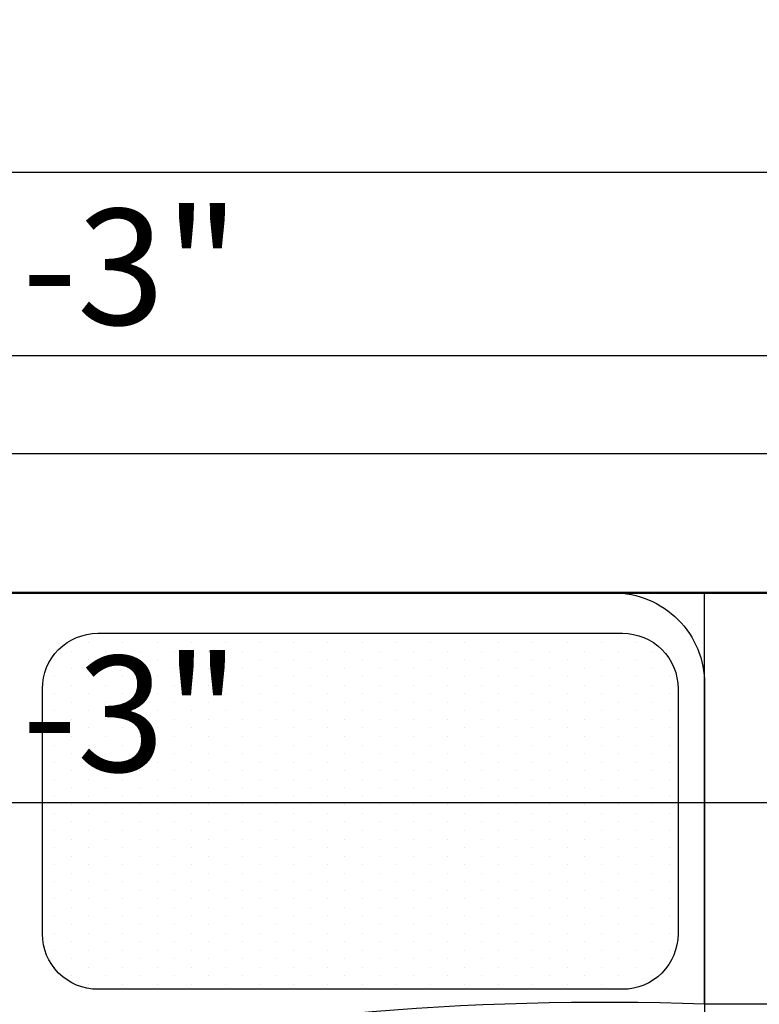
# Model space of a CAD drawing. Units: inches. Extents: x 3064 to 19385, y 846 to 15425.
# Tile 90 of 108: x 7338 to 7370, y 1373 to 1415. Entities that reach past the tile are written whole.
import ezdxf

# ---------------------------------------------------------------- set-up
doc = ezdxf.new("R2010")
doc.units = ezdxf.units.IN
for name, color, linetype, lineweight in [('A-ANNO-DIMS', 2, 'Continuous', 18), ('A-FLOR-FIXT', 9, 'Continuous', 18), ('A-WALL', 7, 'Continuous', 50), ('C-PROP', 6, 'Continuous', 25)]:
    doc.layers.add(name, color=color, linetype=linetype, lineweight=lineweight)
doc.layers.add('BLOCK', color=6, linetype='Continuous')
doc.styles.get("Standard").update_dxf_attribs({"font": 'arial.ttf'})
doc.dimstyles.new('ISO-25', dxfattribs={"dimtxt": 9, "dimasz": 2.5, "dimexe": 1.25, "dimexo": 0.625, "dimtad": 1, "dimdec": 1, "dimlunit": 3, "dimtxsty": 'Standard', "dimcen": 2.5, "dimadec": 0, "dimazin": 0, "dimtfac": 1, "dimtdec": 1, "dimtmove": 0, "dimatfit": 3, "dimfxl": 1, "dimarcsym": 0})

# ---------------------------------------------------------------- blocks, each defined once
blk = doc.blocks.new('*D294')
at = {"layer": 'A-ANNO-DIMS', "color": 0, "lineweight": -2, "transparency": 16777216}
for p, q in [((7240.705, 1396.965), (7240.705, 1401.844)), ((7435.705, 1396.965), (7435.705, 1401.844)), ((7243.205, 1400.594), (7433.205, 1400.594))]:
    blk.add_line(p, q, dxfattribs=at)
at = {"layer": 'A-ANNO-DIMS', "color": 0, "transparency": 16777216}
for points in [[(7243.205, 1401.011), (7243.205, 1400.178), (7240.705, 1400.594)], [(7433.205, 1401.011), (7433.205, 1400.178), (7435.705, 1400.594)]]:
    blk.add_solid(points, dxfattribs=at)
at = {"layer": 'Defpoints', "color": 0, "transparency": 16777216}
for p in [(7435.705, 1400.594), (7240.705, 1396.34), (7435.705, 1396.34)]:
    blk.add_point(p, dxfattribs=at)
at = {"layer": 'A-ANNO-DIMS', "color": 0, "transparency": 16777216, "insert": (7338.205, 1403.774), "char_height": 5, "attachment_point": 5}
blk.add_mtext('16\'-3"', dxfattribs=at)
blk = doc.blocks.new('*D315')
at = {"layer": 'A-ANNO-DIMS', "color": 0, "lineweight": -2, "transparency": 16777216}
for p, q in [((7099.705, 1396.965), (7099.705, 1409.763)), ((7441.705, 1396.965), (7441.705, 1409.763)), ((7102.205, 1408.513), (7439.205, 1408.513))]:
    blk.add_line(p, q, dxfattribs=at)
at = {"layer": 'A-ANNO-DIMS', "color": 0, "transparency": 16777216}
for points in [[(7102.205, 1408.929), (7102.205, 1408.096), (7099.705, 1408.513)], [(7439.205, 1408.929), (7439.205, 1408.096), (7441.705, 1408.513)]]:
    blk.add_solid(points, dxfattribs=at)
at = {"layer": 'Defpoints', "color": 0, "transparency": 16777216}
for p in [(7441.705, 1408.513), (7099.705, 1396.34), (7441.705, 1396.34)]:
    blk.add_point(p, dxfattribs=at)
at = {"layer": 'A-ANNO-DIMS', "color": 0, "transparency": 16777216, "insert": (7270.705, 1411.691), "char_height": 5, "attachment_point": 5}
blk.add_mtext('28\'-6"', dxfattribs=at)
blk = doc.blocks.new('*D290')
at = {"layer": 'A-ANNO-DIMS', "color": 0, "lineweight": -2, "transparency": 16777216}
for p, q in [((7240.705, 1389.715), (7240.705, 1380.039)), ((7435.705, 1389.715), (7435.705, 1380.039)), ((7243.205, 1381.289), (7433.205, 1381.289))]:
    blk.add_line(p, q, dxfattribs=at)
at = {"layer": 'A-ANNO-DIMS', "color": 0, "transparency": 16777216}
for points in [[(7243.205, 1381.705), (7243.205, 1380.872), (7240.705, 1381.289)], [(7433.205, 1381.705), (7433.205, 1380.872), (7435.705, 1381.289)]]:
    blk.add_solid(points, dxfattribs=at)
at = {"layer": 'Defpoints', "color": 0, "transparency": 16777216}
for p in [(7240.705, 1390.34), (7435.705, 1390.34), (7435.705, 1381.289)]:
    blk.add_point(p, dxfattribs=at)
at = {"layer": 'A-ANNO-DIMS', "color": 0, "transparency": 16777216, "insert": (7338.205, 1384.468), "char_height": 5, "attachment_point": 5}
blk.add_mtext('16\'-3"', dxfattribs=at)
blk = doc.blocks.new('*X7')
at = {"color": 0}
for p, q in [((273.75, 456.9375), (273.75, 456.9375)), ((273.9375, 457.03125), (273.9375, 457.03125)), ((274.125, 456.9375), (274.125, 456.9375)), ((274.3125, 457.03125), (274.3125, 457.03125)), ((274.5, 456.9375), (274.5, 456.9375)), ((274.6875, 457.03125), (274.6875, 457.03125)), ((274.875, 456.9375), (274.875, 456.9375)), ((275.0625, 457.03125), (275.0625, 457.03125)), ((275.25, 456.9375), (275.25, 456.9375)), ((275.4375, 457.03125), (275.4375, 457.03125)), ((275.625, 456.9375), (275.625, 456.9375)), ((275.8125, 457.03125), (275.8125, 457.03125)), ((276, 456.9375), (276, 456.9375)), ((276.1875, 457.03125), (276.1875, 457.03125)), ((276.375, 456.9375), (276.375, 456.9375)), ((276.5625, 457.03125), (276.5625, 457.03125)), ((276.75, 456.9375), (276.75, 456.9375)), ((276.9375, 457.03125), (276.9375, 457.03125)), ((277.125, 456.9375), (277.125, 456.9375)), ((277.3125, 457.03125), (277.3125, 457.03125)), ((277.5, 456.9375), (277.5, 456.9375)), ((277.6875, 457.03125), (277.6875, 457.03125)), ((277.875, 456.9375), (277.875, 456.9375)), ((278.0625, 457.03125), (278.0625, 457.03125)), ((278.25, 456.9375), (278.25, 456.9375)), ((278.4375, 457.03125), (278.4375, 457.03125)), ((278.625, 456.9375), (278.625, 456.9375)), ((278.8125, 457.03125), (278.8125, 457.03125)), ((279, 456.9375), (279, 456.9375)), ((279.1875, 457.03125), (279.1875, 457.03125)), ((279.375, 456.9375), (279.375, 456.9375)), ((279.5625, 457.03125), (279.5625, 457.03125)), ((279.75, 456.9375), (279.75, 456.9375)), ((273.5625, 456.84375), (273.5625, 456.84375)), ((273.9375, 456.84375), (273.9375, 456.84375)), ((274.3125, 456.84375), (274.3125, 456.84375)), ((274.6875, 456.84375), (274.6875, 456.84375)), ((275.0625, 456.84375), (275.0625, 456.84375)), ((275.4375, 456.84375), (275.4375, 456.84375)), ((275.8125, 456.84375), (275.8125, 456.84375)), ((276.1875, 456.84375), (276.1875, 456.84375)), ((276.5625, 456.84375), (276.5625, 456.84375)), ((276.9375, 456.84375), (276.9375, 456.84375)), ((277.3125, 456.84375), (277.3125, 456.84375)), ((277.6875, 456.84375), (277.6875, 456.84375)), ((278.0625, 456.84375), (278.0625, 456.84375)), ((278.4375, 456.84375), (278.4375, 456.84375)), ((278.8125, 456.84375), (278.8125, 456.84375)), ((279.1875, 456.84375), (279.1875, 456.84375)), ((279.5625, 456.84375), (279.5625, 456.84375)), ((279.9375, 456.84375), (279.9375, 456.84375)), ((273.375, 456.75), (273.375, 456.75)), ((273.75, 456.75), (273.75, 456.75)), ((274.125, 456.75), (274.125, 456.75)), ((274.5, 456.75), (274.5, 456.75)), ((274.875, 456.75), (274.875, 456.75)), ((275.25, 456.75), (275.25, 456.75)), ((275.625, 456.75), (275.625, 456.75)), ((276, 456.75), (276, 456.75)), ((276.375, 456.75), (276.375, 456.75)), ((276.75, 456.75), (276.75, 456.75)), ((277.125, 456.75), (277.125, 456.75)), ((277.5, 456.75), (277.5, 456.75)), ((277.875, 456.75), (277.875, 456.75)), ((278.25, 456.75), (278.25, 456.75)), ((278.625, 456.75), (278.625, 456.75)), ((279, 456.75), (279, 456.75)), ((279.375, 456.75), (279.375, 456.75)), ((279.75, 456.75), (279.75, 456.75)), ((280.125, 456.75), (280.125, 456.75)), ((273.5625, 456.65625), (273.5625, 456.65625)), ((273.9375, 456.65625), (273.9375, 456.65625)), ((274.3125, 456.65625), (274.3125, 456.65625)), ((274.6875, 456.65625), (274.6875, 456.65625)), ((275.0625, 456.65625), (275.0625, 456.65625)), ((275.4375, 456.65625), (275.4375, 456.65625)), ((275.8125, 456.65625), (275.8125, 456.65625)), ((276.1875, 456.65625), (276.1875, 456.65625)), ((276.5625, 456.65625), (276.5625, 456.65625)), ((276.9375, 456.65625), (276.9375, 456.65625)), ((277.3125, 456.65625), (277.3125, 456.65625)), ((277.6875, 456.65625), (277.6875, 456.65625)), ((278.0625, 456.65625), (278.0625, 456.65625)), ((278.4375, 456.65625), (278.4375, 456.65625)), ((278.8125, 456.65625), (278.8125, 456.65625)), ((279.1875, 456.65625), (279.1875, 456.65625)), ((279.5625, 456.65625), (279.5625, 456.65625)), ((279.9375, 456.65625), (279.9375, 456.65625)), ((273.375, 456.5625), (273.375, 456.5625)), ((273.75, 456.5625), (273.75, 456.5625)), ((274.125, 456.5625), (274.125, 456.5625)), ((274.5, 456.5625), (274.5, 456.5625)), ((274.875, 456.5625), (274.875, 456.5625)), ((275.25, 456.5625), (275.25, 456.5625)), ((275.625, 456.5625), (275.625, 456.5625)), ((276, 456.5625), (276, 456.5625)), ((276.375, 456.5625), (276.375, 456.5625)), ((276.75, 456.5625), (276.75, 456.5625)), ((277.125, 456.5625), (277.125, 456.5625)), ((277.5, 456.5625), (277.5, 456.5625)), ((277.875, 456.5625), (277.875, 456.5625)), ((278.25, 456.5625), (278.25, 456.5625)), ((278.625, 456.5625), (278.625, 456.5625)), ((279, 456.5625), (279, 456.5625)), ((279.375, 456.5625), (279.375, 456.5625)), ((279.75, 456.5625), (279.75, 456.5625)), ((280.125, 456.5625), (280.125, 456.5625)), ((273.5625, 456.46875), (273.5625, 456.46875)), ((273.9375, 456.46875), (273.9375, 456.46875)), ((274.3125, 456.46875), (274.3125, 456.46875)), ((274.6875, 456.46875), (274.6875, 456.46875)), ((275.0625, 456.46875), (275.0625, 456.46875)), ((275.4375, 456.46875), (275.4375, 456.46875)), ((275.8125, 456.46875), (275.8125, 456.46875)), ((276.1875, 456.46875), (276.1875, 456.46875)), ((276.5625, 456.46875), (276.5625, 456.46875)), ((276.9375, 456.46875), (276.9375, 456.46875)), ((277.3125, 456.46875), (277.3125, 456.46875)), ((277.6875, 456.46875), (277.6875, 456.46875)), ((278.0625, 456.46875), (278.0625, 456.46875)), ((278.4375, 456.46875), (278.4375, 456.46875)), ((278.8125, 456.46875), (278.8125, 456.46875)), ((279.1875, 456.46875), (279.1875, 456.46875)), ((279.5625, 456.46875), (279.5625, 456.46875)), ((279.9375, 456.46875), (279.9375, 456.46875)), ((273.375, 456.375), (273.375, 456.375)), ((273.75, 456.375), (273.75, 456.375)), ((274.125, 456.375), (274.125, 456.375)), ((274.5, 456.375), (274.5, 456.375)), ((274.875, 456.375), (274.875, 456.375)), ((275.25, 456.375), (275.25, 456.375)), ((275.625, 456.375), (275.625, 456.375)), ((276, 456.375), (276, 456.375)), ((276.375, 456.375), (276.375, 456.375)), ((276.75, 456.375), (276.75, 456.375)), ((277.125, 456.375), (277.125, 456.375)), ((277.5, 456.375), (277.5, 456.375)), ((277.875, 456.375), (277.875, 456.375)), ((278.25, 456.375), (278.25, 456.375)), ((278.625, 456.375), (278.625, 456.375)), ((279, 456.375), (279, 456.375)), ((279.375, 456.375), (279.375, 456.375)), ((279.75, 456.375), (279.75, 456.375)), ((280.125, 456.375), (280.125, 456.375)), ((273.375, 456.1875), (273.375, 456.1875)), ((273.5625, 456.28125), (273.5625, 456.28125)), ((273.75, 456.1875), (273.75, 456.1875)), ((273.9375, 456.28125), (273.9375, 456.28125)), ((274.125, 456.1875), (274.125, 456.1875)), ((274.3125, 456.28125), (274.3125, 456.28125)), ((274.5, 456.1875), (274.5, 456.1875)), ((274.6875, 456.28125), (274.6875, 456.28125)), ((274.875, 456.1875), (274.875, 456.1875)), ((275.0625, 456.28125), (275.0625, 456.28125)), ((275.25, 456.1875), (275.25, 456.1875)), ((275.4375, 456.28125), (275.4375, 456.28125)), ((275.625, 456.1875), (275.625, 456.1875)), ((275.8125, 456.28125), (275.8125, 456.28125)), ((276, 456.1875), (276, 456.1875)), ((276.1875, 456.28125), (276.1875, 456.28125)), ((276.375, 456.1875), (276.375, 456.1875)), ((276.5625, 456.28125), (276.5625, 456.28125)), ((276.75, 456.1875), (276.75, 456.1875)), ((276.9375, 456.28125), (276.9375, 456.28125)), ((277.125, 456.1875), (277.125, 456.1875)), ((277.3125, 456.28125), (277.3125, 456.28125)), ((277.5, 456.1875), (277.5, 456.1875)), ((277.6875, 456.28125), (277.6875, 456.28125)), ((277.875, 456.1875), (277.875, 456.1875)), ((278.0625, 456.28125), (278.0625, 456.28125)), ((278.25, 456.1875), (278.25, 456.1875)), ((278.4375, 456.28125), (278.4375, 456.28125)), ((278.625, 456.1875), (278.625, 456.1875)), ((278.8125, 456.28125), (278.8125, 456.28125)), ((279, 456.1875), (279, 456.1875)), ((279.1875, 456.28125), (279.1875, 456.28125)), ((279.375, 456.1875), (279.375, 456.1875)), ((279.5625, 456.28125), (279.5625, 456.28125)), ((279.75, 456.1875), (279.75, 456.1875)), ((279.9375, 456.28125), (279.9375, 456.28125)), ((280.125, 456.1875), (280.125, 456.1875)), ((273.5625, 456.09375), (273.5625, 456.09375)), ((273.9375, 456.09375), (273.9375, 456.09375)), ((274.3125, 456.09375), (274.3125, 456.09375)), ((274.6875, 456.09375), (274.6875, 456.09375)), ((275.0625, 456.09375), (275.0625, 456.09375)), ((275.4375, 456.09375), (275.4375, 456.09375)), ((275.8125, 456.09375), (275.8125, 456.09375)), ((276.1875, 456.09375), (276.1875, 456.09375)), ((276.5625, 456.09375), (276.5625, 456.09375)), ((276.9375, 456.09375), (276.9375, 456.09375)), ((277.3125, 456.09375), (277.3125, 456.09375)), ((277.6875, 456.09375), (277.6875, 456.09375)), ((278.0625, 456.09375), (278.0625, 456.09375)), ((278.4375, 456.09375), (278.4375, 456.09375)), ((278.8125, 456.09375), (278.8125, 456.09375)), ((279.1875, 456.09375), (279.1875, 456.09375)), ((279.5625, 456.09375), (279.5625, 456.09375)), ((279.9375, 456.09375), (279.9375, 456.09375)), ((273.375, 456), (273.375, 456)), ((273.75, 456), (273.75, 456)), ((274.125, 456), (274.125, 456)), ((274.5, 456), (274.5, 456)), ((274.875, 456), (274.875, 456)), ((275.25, 456), (275.25, 456)), ((275.625, 456), (275.625, 456)), ((276, 456), (276, 456)), ((276.375, 456), (276.375, 456)), ((276.75, 456), (276.75, 456)), ((277.125, 456), (277.125, 456)), ((277.5, 456), (277.5, 456)), ((277.875, 456), (277.875, 456)), ((278.25, 456), (278.25, 456)), ((278.625, 456), (278.625, 456)), ((279, 456), (279, 456)), ((279.375, 456), (279.375, 456)), ((279.75, 456), (279.75, 456)), ((280.125, 456), (280.125, 456)), ((273.5625, 455.90625), (273.5625, 455.90625)), ((273.9375, 455.90625), (273.9375, 455.90625)), ((274.3125, 455.90625), (274.3125, 455.90625)), ((274.6875, 455.90625), (274.6875, 455.90625)), ((275.0625, 455.90625), (275.0625, 455.90625)), ((275.4375, 455.90625), (275.4375, 455.90625)), ((275.8125, 455.90625), (275.8125, 455.90625)), ((276.1875, 455.90625), (276.1875, 455.90625)), ((276.5625, 455.90625), (276.5625, 455.90625)), ((276.9375, 455.90625), (276.9375, 455.90625)), ((277.3125, 455.90625), (277.3125, 455.90625)), ((277.6875, 455.90625), (277.6875, 455.90625)), ((278.0625, 455.90625), (278.0625, 455.90625)), ((278.4375, 455.90625), (278.4375, 455.90625)), ((278.8125, 455.90625), (278.8125, 455.90625)), ((279.1875, 455.90625), (279.1875, 455.90625)), ((279.5625, 455.90625), (279.5625, 455.90625)), ((279.9375, 455.90625), (279.9375, 455.90625)), ((273.375, 455.8125), (273.375, 455.8125)), ((273.75, 455.8125), (273.75, 455.8125)), ((274.125, 455.8125), (274.125, 455.8125)), ((274.5, 455.8125), (274.5, 455.8125)), ((274.875, 455.8125), (274.875, 455.8125)), ((275.25, 455.8125), (275.25, 455.8125)), ((275.625, 455.8125), (275.625, 455.8125)), ((276, 455.8125), (276, 455.8125)), ((276.375, 455.8125), (276.375, 455.8125)), ((276.75, 455.8125), (276.75, 455.8125)), ((277.125, 455.8125), (277.125, 455.8125)), ((277.5, 455.8125), (277.5, 455.8125)), ((277.875, 455.8125), (277.875, 455.8125)), ((278.25, 455.8125), (278.25, 455.8125)), ((278.625, 455.8125), (278.625, 455.8125)), ((279, 455.8125), (279, 455.8125)), ((279.375, 455.8125), (279.375, 455.8125)), ((279.75, 455.8125), (279.75, 455.8125)), ((280.125, 455.8125), (280.125, 455.8125)), ((273.5625, 455.71875), (273.5625, 455.71875)), ((273.9375, 455.71875), (273.9375, 455.71875)), ((274.3125, 455.71875), (274.3125, 455.71875)), ((274.6875, 455.71875), (274.6875, 455.71875)), ((275.0625, 455.71875), (275.0625, 455.71875)), ((275.4375, 455.71875), (275.4375, 455.71875)), ((275.8125, 455.71875), (275.8125, 455.71875)), ((276.1875, 455.71875), (276.1875, 455.71875)), ((276.5625, 455.71875), (276.5625, 455.71875)), ((276.9375, 455.71875), (276.9375, 455.71875)), ((277.3125, 455.71875), (277.3125, 455.71875)), ((277.6875, 455.71875), (277.6875, 455.71875)), ((278.0625, 455.71875), (278.0625, 455.71875)), ((278.4375, 455.71875), (278.4375, 455.71875)), ((278.8125, 455.71875), (278.8125, 455.71875)), ((279.1875, 455.71875), (279.1875, 455.71875)), ((279.5625, 455.71875), (279.5625, 455.71875)), ((279.9375, 455.71875), (279.9375, 455.71875)), ((273.375, 455.625), (273.375, 455.625)), ((273.5625, 455.53125), (273.5625, 455.53125)), ((273.75, 455.625), (273.75, 455.625)), ((273.9375, 455.53125), (273.9375, 455.53125)), ((274.125, 455.625), (274.125, 455.625)), ((274.3125, 455.53125), (274.3125, 455.53125)), ((274.5, 455.625), (274.5, 455.625)), ((274.6875, 455.53125), (274.6875, 455.53125)), ((274.875, 455.625), (274.875, 455.625)), ((275.0625, 455.53125), (275.0625, 455.53125)), ((275.25, 455.625), (275.25, 455.625)), ((275.4375, 455.53125), (275.4375, 455.53125)), ((275.625, 455.625), (275.625, 455.625)), ((275.8125, 455.53125), (275.8125, 455.53125)), ((276, 455.625), (276, 455.625)), ((276.1875, 455.53125), (276.1875, 455.53125)), ((276.375, 455.625), (276.375, 455.625)), ((276.5625, 455.53125), (276.5625, 455.53125)), ((276.75, 455.625), (276.75, 455.625)), ((276.9375, 455.53125), (276.9375, 455.53125)), ((277.125, 455.625), (277.125, 455.625)), ((277.3125, 455.53125), (277.3125, 455.53125)), ((277.5, 455.625), (277.5, 455.625)), ((277.6875, 455.53125), (277.6875, 455.53125)), ((277.875, 455.625), (277.875, 455.625)), ((278.0625, 455.53125), (278.0625, 455.53125)), ((278.25, 455.625), (278.25, 455.625)), ((278.4375, 455.53125), (278.4375, 455.53125)), ((278.625, 455.625), (278.625, 455.625)), ((278.8125, 455.53125), (278.8125, 455.53125)), ((279, 455.625), (279, 455.625)), ((279.1875, 455.53125), (279.1875, 455.53125)), ((279.375, 455.625), (279.375, 455.625)), ((279.5625, 455.53125), (279.5625, 455.53125)), ((279.75, 455.625), (279.75, 455.625)), ((279.9375, 455.53125), (279.9375, 455.53125)), ((280.125, 455.625), (280.125, 455.625)), ((273.375, 455.4375), (273.375, 455.4375)), ((273.75, 455.4375), (273.75, 455.4375)), ((274.125, 455.4375), (274.125, 455.4375)), ((274.5, 455.4375), (274.5, 455.4375)), ((274.875, 455.4375), (274.875, 455.4375)), ((275.25, 455.4375), (275.25, 455.4375)), ((275.625, 455.4375), (275.625, 455.4375)), ((276, 455.4375), (276, 455.4375)), ((276.375, 455.4375), (276.375, 455.4375)), ((276.75, 455.4375), (276.75, 455.4375)), ((277.125, 455.4375), (277.125, 455.4375)), ((277.5, 455.4375), (277.5, 455.4375)), ((277.875, 455.4375), (277.875, 455.4375)), ((278.25, 455.4375), (278.25, 455.4375)), ((278.625, 455.4375), (278.625, 455.4375)), ((279, 455.4375), (279, 455.4375)), ((279.375, 455.4375), (279.375, 455.4375)), ((279.75, 455.4375), (279.75, 455.4375)), ((280.125, 455.4375), (280.125, 455.4375)), ((273.5625, 455.34375), (273.5625, 455.34375)), ((273.9375, 455.34375), (273.9375, 455.34375)), ((274.3125, 455.34375), (274.3125, 455.34375)), ((274.6875, 455.34375), (274.6875, 455.34375)), ((275.0625, 455.34375), (275.0625, 455.34375)), ((275.4375, 455.34375), (275.4375, 455.34375)), ((275.8125, 455.34375), (275.8125, 455.34375)), ((276.1875, 455.34375), (276.1875, 455.34375)), ((276.5625, 455.34375), (276.5625, 455.34375)), ((276.9375, 455.34375), (276.9375, 455.34375)), ((277.3125, 455.34375), (277.3125, 455.34375)), ((277.6875, 455.34375), (277.6875, 455.34375)), ((278.0625, 455.34375), (278.0625, 455.34375)), ((278.4375, 455.34375), (278.4375, 455.34375)), ((278.8125, 455.34375), (278.8125, 455.34375)), ((279.1875, 455.34375), (279.1875, 455.34375)), ((279.5625, 455.34375), (279.5625, 455.34375)), ((279.9375, 455.34375), (279.9375, 455.34375)), ((273.375, 455.25), (273.375, 455.25)), ((273.75, 455.25), (273.75, 455.25)), ((274.125, 455.25), (274.125, 455.25)), ((274.5, 455.25), (274.5, 455.25)), ((274.875, 455.25), (274.875, 455.25)), ((275.25, 455.25), (275.25, 455.25)), ((275.625, 455.25), (275.625, 455.25)), ((276, 455.25), (276, 455.25)), ((276.375, 455.25), (276.375, 455.25)), ((276.75, 455.25), (276.75, 455.25)), ((277.125, 455.25), (277.125, 455.25)), ((277.5, 455.25), (277.5, 455.25)), ((277.875, 455.25), (277.875, 455.25)), ((278.25, 455.25), (278.25, 455.25)), ((278.625, 455.25), (278.625, 455.25)), ((279, 455.25), (279, 455.25)), ((279.375, 455.25), (279.375, 455.25)), ((279.75, 455.25), (279.75, 455.25)), ((280.125, 455.25), (280.125, 455.25)), ((273.5625, 455.15625), (273.5625, 455.15625)), ((273.9375, 455.15625), (273.9375, 455.15625)), ((274.3125, 455.15625), (274.3125, 455.15625)), ((274.6875, 455.15625), (274.6875, 455.15625)), ((275.0625, 455.15625), (275.0625, 455.15625)), ((275.4375, 455.15625), (275.4375, 455.15625)), ((275.8125, 455.15625), (275.8125, 455.15625)), ((276.1875, 455.15625), (276.1875, 455.15625)), ((276.5625, 455.15625), (276.5625, 455.15625)), ((276.9375, 455.15625), (276.9375, 455.15625)), ((277.3125, 455.15625), (277.3125, 455.15625)), ((277.6875, 455.15625), (277.6875, 455.15625)), ((278.0625, 455.15625), (278.0625, 455.15625)), ((278.4375, 455.15625), (278.4375, 455.15625)), ((278.8125, 455.15625), (278.8125, 455.15625)), ((279.1875, 455.15625), (279.1875, 455.15625)), ((279.5625, 455.15625), (279.5625, 455.15625)), ((279.9375, 455.15625), (279.9375, 455.15625)), ((273.375, 455.0625), (273.375, 455.0625)), ((273.75, 455.0625), (273.75, 455.0625)), ((274.125, 455.0625), (274.125, 455.0625)), ((274.5, 455.0625), (274.5, 455.0625)), ((274.875, 455.0625), (274.875, 455.0625)), ((275.25, 455.0625), (275.25, 455.0625)), ((275.625, 455.0625), (275.625, 455.0625)), ((276, 455.0625), (276, 455.0625)), ((276.375, 455.0625), (276.375, 455.0625)), ((276.75, 455.0625), (276.75, 455.0625)), ((277.125, 455.0625), (277.125, 455.0625)), ((277.5, 455.0625), (277.5, 455.0625)), ((277.875, 455.0625), (277.875, 455.0625)), ((278.25, 455.0625), (278.25, 455.0625)), ((278.625, 455.0625), (278.625, 455.0625)), ((279, 455.0625), (279, 455.0625)), ((279.375, 455.0625), (279.375, 455.0625)), ((279.75, 455.0625), (279.75, 455.0625)), ((280.125, 455.0625), (280.125, 455.0625)), ((273.5625, 454.96875), (273.5625, 454.96875)), ((273.9375, 454.96875), (273.9375, 454.96875)), ((274.3125, 454.96875), (274.3125, 454.96875)), ((274.6875, 454.96875), (274.6875, 454.96875)), ((275.0625, 454.96875), (275.0625, 454.96875)), ((275.4375, 454.96875), (275.4375, 454.96875)), ((275.8125, 454.96875), (275.8125, 454.96875)), ((276.1875, 454.96875), (276.1875, 454.96875)), ((276.5625, 454.96875), (276.5625, 454.96875)), ((276.9375, 454.96875), (276.9375, 454.96875)), ((277.3125, 454.96875), (277.3125, 454.96875)), ((277.6875, 454.96875), (277.6875, 454.96875)), ((278.0625, 454.96875), (278.0625, 454.96875)), ((278.4375, 454.96875), (278.4375, 454.96875)), ((278.8125, 454.96875), (278.8125, 454.96875)), ((279.1875, 454.96875), (279.1875, 454.96875)), ((279.5625, 454.96875), (279.5625, 454.96875)), ((279.9375, 454.96875), (279.9375, 454.96875)), ((273.375, 454.875), (273.375, 454.875)), ((273.5625, 454.78125), (273.5625, 454.78125)), ((273.75, 454.875), (273.75, 454.875)), ((273.9375, 454.78125), (273.9375, 454.78125)), ((274.125, 454.875), (274.125, 454.875)), ((274.3125, 454.78125), (274.3125, 454.78125)), ((274.5, 454.875), (274.5, 454.875)), ((274.6875, 454.78125), (274.6875, 454.78125)), ((274.875, 454.875), (274.875, 454.875)), ((275.0625, 454.78125), (275.0625, 454.78125)), ((275.25, 454.875), (275.25, 454.875)), ((275.4375, 454.78125), (275.4375, 454.78125)), ((275.625, 454.875), (275.625, 454.875)), ((275.8125, 454.78125), (275.8125, 454.78125)), ((276, 454.875), (276, 454.875)), ((276.1875, 454.78125), (276.1875, 454.78125)), ((276.375, 454.875), (276.375, 454.875)), ((276.5625, 454.78125), (276.5625, 454.78125)), ((276.75, 454.875), (276.75, 454.875)), ((276.9375, 454.78125), (276.9375, 454.78125)), ((277.125, 454.875), (277.125, 454.875)), ((277.3125, 454.78125), (277.3125, 454.78125)), ((277.5, 454.875), (277.5, 454.875)), ((277.6875, 454.78125), (277.6875, 454.78125)), ((277.875, 454.875), (277.875, 454.875)), ((278.0625, 454.78125), (278.0625, 454.78125)), ((278.25, 454.875), (278.25, 454.875)), ((278.4375, 454.78125), (278.4375, 454.78125)), ((278.625, 454.875), (278.625, 454.875)), ((278.8125, 454.78125), (278.8125, 454.78125)), ((279, 454.875), (279, 454.875)), ((279.1875, 454.78125), (279.1875, 454.78125)), ((279.375, 454.875), (279.375, 454.875)), ((279.5625, 454.78125), (279.5625, 454.78125)), ((279.75, 454.875), (279.75, 454.875)), ((279.9375, 454.78125), (279.9375, 454.78125)), ((280.125, 454.875), (280.125, 454.875)), ((273.375, 454.6875), (273.375, 454.6875)), ((273.75, 454.6875), (273.75, 454.6875)), ((274.125, 454.6875), (274.125, 454.6875)), ((274.5, 454.6875), (274.5, 454.6875)), ((274.875, 454.6875), (274.875, 454.6875)), ((275.25, 454.6875), (275.25, 454.6875)), ((275.625, 454.6875), (275.625, 454.6875)), ((276, 454.6875), (276, 454.6875)), ((276.375, 454.6875), (276.375, 454.6875)), ((276.75, 454.6875), (276.75, 454.6875)), ((277.125, 454.6875), (277.125, 454.6875)), ((277.5, 454.6875), (277.5, 454.6875)), ((277.875, 454.6875), (277.875, 454.6875)), ((278.25, 454.6875), (278.25, 454.6875)), ((278.625, 454.6875), (278.625, 454.6875)), ((279, 454.6875), (279, 454.6875)), ((279.375, 454.6875), (279.375, 454.6875)), ((279.75, 454.6875), (279.75, 454.6875)), ((280.125, 454.6875), (280.125, 454.6875)), ((273.5625, 454.59375), (273.5625, 454.59375)), ((273.9375, 454.59375), (273.9375, 454.59375)), ((274.3125, 454.59375), (274.3125, 454.59375)), ((274.6875, 454.59375), (274.6875, 454.59375)), ((275.0625, 454.59375), (275.0625, 454.59375)), ((275.4375, 454.59375), (275.4375, 454.59375)), ((275.8125, 454.59375), (275.8125, 454.59375)), ((276.1875, 454.59375), (276.1875, 454.59375)), ((276.5625, 454.59375), (276.5625, 454.59375)), ((276.9375, 454.59375), (276.9375, 454.59375)), ((277.3125, 454.59375), (277.3125, 454.59375)), ((277.6875, 454.59375), (277.6875, 454.59375)), ((278.0625, 454.59375), (278.0625, 454.59375)), ((278.4375, 454.59375), (278.4375, 454.59375)), ((278.8125, 454.59375), (278.8125, 454.59375)), ((279.1875, 454.59375), (279.1875, 454.59375)), ((279.5625, 454.59375), (279.5625, 454.59375)), ((279.9375, 454.59375), (279.9375, 454.59375)), ((273.375, 454.5), (273.375, 454.5)), ((273.75, 454.5), (273.75, 454.5)), ((274.125, 454.5), (274.125, 454.5)), ((274.5, 454.5), (274.5, 454.5)), ((274.875, 454.5), (274.875, 454.5)), ((275.25, 454.5), (275.25, 454.5)), ((275.625, 454.5), (275.625, 454.5)), ((276, 454.5), (276, 454.5)), ((276.375, 454.5), (276.375, 454.5)), ((276.75, 454.5), (276.75, 454.5)), ((277.125, 454.5), (277.125, 454.5)), ((277.5, 454.5), (277.5, 454.5)), ((277.875, 454.5), (277.875, 454.5)), ((278.25, 454.5), (278.25, 454.5)), ((278.625, 454.5), (278.625, 454.5)), ((279, 454.5), (279, 454.5)), ((279.375, 454.5), (279.375, 454.5)), ((279.75, 454.5), (279.75, 454.5)), ((280.125, 454.5), (280.125, 454.5)), ((273.5625, 454.40625), (273.5625, 454.40625)), ((273.9375, 454.40625), (273.9375, 454.40625)), ((274.3125, 454.40625), (274.3125, 454.40625)), ((274.6875, 454.40625), (274.6875, 454.40625)), ((275.0625, 454.40625), (275.0625, 454.40625)), ((275.4375, 454.40625), (275.4375, 454.40625)), ((275.8125, 454.40625), (275.8125, 454.40625)), ((276.1875, 454.40625), (276.1875, 454.40625)), ((276.5625, 454.40625), (276.5625, 454.40625)), ((276.9375, 454.40625), (276.9375, 454.40625)), ((277.3125, 454.40625), (277.3125, 454.40625)), ((277.6875, 454.40625), (277.6875, 454.40625)), ((278.0625, 454.40625), (278.0625, 454.40625)), ((278.4375, 454.40625), (278.4375, 454.40625)), ((278.8125, 454.40625), (278.8125, 454.40625)), ((279.1875, 454.40625), (279.1875, 454.40625)), ((279.5625, 454.40625), (279.5625, 454.40625)), ((279.9375, 454.40625), (279.9375, 454.40625)), ((273.375, 454.3125), (273.375, 454.3125)), ((273.75, 454.3125), (273.75, 454.3125)), ((274.125, 454.3125), (274.125, 454.3125)), ((274.5, 454.3125), (274.5, 454.3125)), ((274.875, 454.3125), (274.875, 454.3125)), ((275.25, 454.3125), (275.25, 454.3125)), ((275.625, 454.3125), (275.625, 454.3125)), ((276, 454.3125), (276, 454.3125)), ((276.375, 454.3125), (276.375, 454.3125)), ((276.75, 454.3125), (276.75, 454.3125)), ((277.125, 454.3125), (277.125, 454.3125)), ((277.5, 454.3125), (277.5, 454.3125)), ((277.875, 454.3125), (277.875, 454.3125)), ((278.25, 454.3125), (278.25, 454.3125)), ((278.625, 454.3125), (278.625, 454.3125)), ((279, 454.3125), (279, 454.3125)), ((279.375, 454.3125), (279.375, 454.3125)), ((279.75, 454.3125), (279.75, 454.3125)), ((280.125, 454.3125), (280.125, 454.3125)), ((273.5625, 454.21875), (273.5625, 454.21875)), ((273.9375, 454.21875), (273.9375, 454.21875)), ((274.3125, 454.21875), (274.3125, 454.21875)), ((274.6875, 454.21875), (274.6875, 454.21875)), ((275.0625, 454.21875), (275.0625, 454.21875)), ((275.4375, 454.21875), (275.4375, 454.21875)), ((275.8125, 454.21875), (275.8125, 454.21875)), ((276.1875, 454.21875), (276.1875, 454.21875)), ((276.5625, 454.21875), (276.5625, 454.21875)), ((276.9375, 454.21875), (276.9375, 454.21875)), ((277.3125, 454.21875), (277.3125, 454.21875)), ((277.6875, 454.21875), (277.6875, 454.21875)), ((278.0625, 454.21875), (278.0625, 454.21875)), ((278.4375, 454.21875), (278.4375, 454.21875)), ((278.8125, 454.21875), (278.8125, 454.21875)), ((279.1875, 454.21875), (279.1875, 454.21875)), ((279.5625, 454.21875), (279.5625, 454.21875)), ((279.9375, 454.21875), (279.9375, 454.21875)), ((273.375, 454.125), (273.375, 454.125)), ((273.5625, 454.03125), (273.5625, 454.03125)), ((273.75, 454.125), (273.75, 454.125)), ((273.9375, 454.03125), (273.9375, 454.03125)), ((274.125, 454.125), (274.125, 454.125)), ((274.3125, 454.03125), (274.3125, 454.03125)), ((274.5, 454.125), (274.5, 454.125)), ((274.6875, 454.03125), (274.6875, 454.03125)), ((274.875, 454.125), (274.875, 454.125)), ((275.0625, 454.03125), (275.0625, 454.03125)), ((275.25, 454.125), (275.25, 454.125)), ((275.4375, 454.03125), (275.4375, 454.03125)), ((275.625, 454.125), (275.625, 454.125)), ((275.8125, 454.03125), (275.8125, 454.03125)), ((276, 454.125), (276, 454.125)), ((276.1875, 454.03125), (276.1875, 454.03125)), ((276.375, 454.125), (276.375, 454.125)), ((276.5625, 454.03125), (276.5625, 454.03125)), ((276.75, 454.125), (276.75, 454.125)), ((276.9375, 454.03125), (276.9375, 454.03125)), ((277.125, 454.125), (277.125, 454.125)), ((277.3125, 454.03125), (277.3125, 454.03125)), ((277.5, 454.125), (277.5, 454.125)), ((277.6875, 454.03125), (277.6875, 454.03125)), ((277.875, 454.125), (277.875, 454.125)), ((278.0625, 454.03125), (278.0625, 454.03125)), ((278.25, 454.125), (278.25, 454.125)), ((278.4375, 454.03125), (278.4375, 454.03125)), ((278.625, 454.125), (278.625, 454.125)), ((278.8125, 454.03125), (278.8125, 454.03125)), ((279, 454.125), (279, 454.125)), ((279.1875, 454.03125), (279.1875, 454.03125)), ((279.375, 454.125), (279.375, 454.125)), ((279.5625, 454.03125), (279.5625, 454.03125)), ((279.75, 454.125), (279.75, 454.125)), ((279.9375, 454.03125), (279.9375, 454.03125)), ((280.125, 454.125), (280.125, 454.125)), ((273.375, 453.9375), (273.375, 453.9375)), ((273.75, 453.9375), (273.75, 453.9375)), ((274.125, 453.9375), (274.125, 453.9375)), ((274.5, 453.9375), (274.5, 453.9375)), ((274.875, 453.9375), (274.875, 453.9375)), ((275.25, 453.9375), (275.25, 453.9375)), ((275.625, 453.9375), (275.625, 453.9375)), ((276, 453.9375), (276, 453.9375)), ((276.375, 453.9375), (276.375, 453.9375)), ((276.75, 453.9375), (276.75, 453.9375)), ((277.125, 453.9375), (277.125, 453.9375)), ((277.5, 453.9375), (277.5, 453.9375)), ((277.875, 453.9375), (277.875, 453.9375)), ((278.25, 453.9375), (278.25, 453.9375)), ((278.625, 453.9375), (278.625, 453.9375)), ((279, 453.9375), (279, 453.9375)), ((279.375, 453.9375), (279.375, 453.9375)), ((279.75, 453.9375), (279.75, 453.9375)), ((280.125, 453.9375), (280.125, 453.9375)), ((273.5625, 453.84375), (273.5625, 453.84375)), ((273.9375, 453.84375), (273.9375, 453.84375)), ((274.3125, 453.84375), (274.3125, 453.84375)), ((274.6875, 453.84375), (274.6875, 453.84375)), ((275.0625, 453.84375), (275.0625, 453.84375)), ((275.4375, 453.84375), (275.4375, 453.84375)), ((275.8125, 453.84375), (275.8125, 453.84375)), ((276.1875, 453.84375), (276.1875, 453.84375)), ((276.5625, 453.84375), (276.5625, 453.84375)), ((276.9375, 453.84375), (276.9375, 453.84375)), ((277.3125, 453.84375), (277.3125, 453.84375)), ((277.6875, 453.84375), (277.6875, 453.84375)), ((278.0625, 453.84375), (278.0625, 453.84375)), ((278.4375, 453.84375), (278.4375, 453.84375)), ((278.8125, 453.84375), (278.8125, 453.84375)), ((279.1875, 453.84375), (279.1875, 453.84375)), ((279.5625, 453.84375), (279.5625, 453.84375)), ((279.9375, 453.84375), (279.9375, 453.84375)), ((273.375, 453.75), (273.375, 453.75)), ((273.75, 453.75), (273.75, 453.75)), ((274.125, 453.75), (274.125, 453.75)), ((274.5, 453.75), (274.5, 453.75)), ((274.875, 453.75), (274.875, 453.75)), ((275.25, 453.75), (275.25, 453.75)), ((275.625, 453.75), (275.625, 453.75)), ((276, 453.75), (276, 453.75)), ((276.375, 453.75), (276.375, 453.75)), ((276.75, 453.75), (276.75, 453.75)), ((277.125, 453.75), (277.125, 453.75)), ((277.5, 453.75), (277.5, 453.75)), ((277.875, 453.75), (277.875, 453.75)), ((278.25, 453.75), (278.25, 453.75)), ((278.625, 453.75), (278.625, 453.75)), ((279, 453.75), (279, 453.75)), ((279.375, 453.75), (279.375, 453.75)), ((279.75, 453.75), (279.75, 453.75)), ((280.125, 453.75), (280.125, 453.75)), ((273.5625, 453.65625), (273.5625, 453.65625)), ((273.9375, 453.65625), (273.9375, 453.65625)), ((274.3125, 453.65625), (274.3125, 453.65625)), ((274.6875, 453.65625), (274.6875, 453.65625)), ((275.0625, 453.65625), (275.0625, 453.65625)), ((275.4375, 453.65625), (275.4375, 453.65625)), ((275.8125, 453.65625), (275.8125, 453.65625)), ((276.1875, 453.65625), (276.1875, 453.65625)), ((276.5625, 453.65625), (276.5625, 453.65625)), ((276.9375, 453.65625), (276.9375, 453.65625)), ((277.3125, 453.65625), (277.3125, 453.65625)), ((277.6875, 453.65625), (277.6875, 453.65625)), ((278.0625, 453.65625), (278.0625, 453.65625)), ((278.4375, 453.65625), (278.4375, 453.65625)), ((278.8125, 453.65625), (278.8125, 453.65625)), ((279.1875, 453.65625), (279.1875, 453.65625)), ((279.5625, 453.65625), (279.5625, 453.65625)), ((279.9375, 453.65625), (279.9375, 453.65625)), ((273.375, 453.5625), (273.375, 453.5625)), ((273.75, 453.5625), (273.75, 453.5625)), ((274.125, 453.5625), (274.125, 453.5625)), ((274.5, 453.5625), (274.5, 453.5625)), ((274.875, 453.5625), (274.875, 453.5625)), ((275.25, 453.5625), (275.25, 453.5625)), ((275.625, 453.5625), (275.625, 453.5625)), ((276, 453.5625), (276, 453.5625)), ((276.375, 453.5625), (276.375, 453.5625)), ((276.75, 453.5625), (276.75, 453.5625)), ((277.125, 453.5625), (277.125, 453.5625)), ((277.5, 453.5625), (277.5, 453.5625)), ((277.875, 453.5625), (277.875, 453.5625)), ((278.25, 453.5625), (278.25, 453.5625)), ((278.625, 453.5625), (278.625, 453.5625)), ((279, 453.5625), (279, 453.5625)), ((279.375, 453.5625), (279.375, 453.5625)), ((279.75, 453.5625), (279.75, 453.5625)), ((280.125, 453.5625), (280.125, 453.5625)), ((273.375, 453.375), (273.375, 453.375)), ((273.5625, 453.46875), (273.5625, 453.46875)), ((273.75, 453.375), (273.75, 453.375)), ((273.9375, 453.46875), (273.9375, 453.46875)), ((274.125, 453.375), (274.125, 453.375)), ((274.3125, 453.46875), (274.3125, 453.46875)), ((274.5, 453.375), (274.5, 453.375)), ((274.6875, 453.46875), (274.6875, 453.46875)), ((274.875, 453.375), (274.875, 453.375)), ((275.0625, 453.46875), (275.0625, 453.46875)), ((275.25, 453.375), (275.25, 453.375)), ((275.4375, 453.46875), (275.4375, 453.46875)), ((275.625, 453.375), (275.625, 453.375)), ((275.8125, 453.46875), (275.8125, 453.46875)), ((276, 453.375), (276, 453.375)), ((276.1875, 453.46875), (276.1875, 453.46875)), ((276.375, 453.375), (276.375, 453.375)), ((276.5625, 453.46875), (276.5625, 453.46875)), ((276.75, 453.375), (276.75, 453.375)), ((276.9375, 453.46875), (276.9375, 453.46875)), ((277.125, 453.375), (277.125, 453.375)), ((277.3125, 453.46875), (277.3125, 453.46875)), ((277.5, 453.375), (277.5, 453.375)), ((277.6875, 453.46875), (277.6875, 453.46875)), ((277.875, 453.375), (277.875, 453.375)), ((278.0625, 453.46875), (278.0625, 453.46875)), ((278.25, 453.375), (278.25, 453.375)), ((278.4375, 453.46875), (278.4375, 453.46875)), ((278.625, 453.375), (278.625, 453.375)), ((278.8125, 453.46875), (278.8125, 453.46875)), ((279, 453.375), (279, 453.375)), ((279.1875, 453.46875), (279.1875, 453.46875)), ((279.375, 453.375), (279.375, 453.375)), ((279.5625, 453.46875), (279.5625, 453.46875)), ((279.75, 453.375), (279.75, 453.375)), ((279.9375, 453.46875), (279.9375, 453.46875)), ((273.5625, 453.28125), (273.5625, 453.28125)), ((273.9375, 453.28125), (273.9375, 453.28125)), ((274.3125, 453.28125), (274.3125, 453.28125)), ((274.6875, 453.28125), (274.6875, 453.28125)), ((275.0625, 453.28125), (275.0625, 453.28125)), ((275.4375, 453.28125), (275.4375, 453.28125)), ((275.8125, 453.28125), (275.8125, 453.28125)), ((276.1875, 453.28125), (276.1875, 453.28125)), ((276.5625, 453.28125), (276.5625, 453.28125)), ((276.9375, 453.28125), (276.9375, 453.28125)), ((277.3125, 453.28125), (277.3125, 453.28125)), ((277.6875, 453.28125), (277.6875, 453.28125)), ((278.0625, 453.28125), (278.0625, 453.28125)), ((278.4375, 453.28125), (278.4375, 453.28125)), ((278.8125, 453.28125), (278.8125, 453.28125)), ((279.1875, 453.28125), (279.1875, 453.28125)), ((279.5625, 453.28125), (279.5625, 453.28125)), ((279.9375, 453.28125), (279.9375, 453.28125)), ((273.75, 453.1875), (273.75, 453.1875)), ((274.125, 453.1875), (274.125, 453.1875)), ((274.5, 453.1875), (274.5, 453.1875)), ((274.875, 453.1875), (274.875, 453.1875)), ((275.25, 453.1875), (275.25, 453.1875)), ((275.625, 453.1875), (275.625, 453.1875)), ((276, 453.1875), (276, 453.1875)), ((276.375, 453.1875), (276.375, 453.1875)), ((276.75, 453.1875), (276.75, 453.1875)), ((277.125, 453.1875), (277.125, 453.1875)), ((277.5, 453.1875), (277.5, 453.1875)), ((277.875, 453.1875), (277.875, 453.1875)), ((278.25, 453.1875), (278.25, 453.1875)), ((278.625, 453.1875), (278.625, 453.1875)), ((279, 453.1875), (279, 453.1875)), ((279.375, 453.1875), (279.375, 453.1875)), ((279.75, 453.1875), (279.75, 453.1875))]:
    blk.add_line(p, q, dxfattribs=at)
blk = doc.blocks.new('A$C52E67D0D')
at = {"layer": 'BLOCK'}
for points in [[(1901, 0), (601, 0, -0.414214), (501, 100), (501, 1700, -0.414214), (601, 1800), (1901, 1800, -0.414214), (2001, 1700), (2001, 100, -0.414214)], [(1911, 1365.1), (1335, 1365.1, -0.414214), (1274.2, 1425.9), (1274.2, 1694.8, -0.414214), (1335, 1755.7), (1911, 1755.7, -0.414214), (1971.8, 1694.8), (1971.8, 1425.9, -0.414214)]]:
    blk.add_lwpolyline(points, format="xyb", close=True, dxfattribs=at)
blk.add_lwpolyline([(2001, 1348.6), (2001, 1799.6), (2502, 1799.6), (2502, 1348.6)], close=True, dxfattribs=at)
blk.add_arc((1888.6, -1664.5), 3015.3, 87.8642, 117.4001, dxfattribs=at)
at = {"layer": 'BLOCK', "xscale": 100, "yscale": 100, "zscale": 100}
blk.add_blockref('*X7', (-26050, -43948.2), dxfattribs=at)

msp = doc.modelspace()

# ---------------------------------------------------------------- linework, layer by layer
at = {"layer": 'A-WALL'}
msp.add_line((7435.705, 1390.34), (7240.705, 1390.34), dxfattribs=at)
at = {"layer": 'C-PROP'}
msp.add_line((7441.705, 1396.34), (7099.705, 1396.34), dxfattribs=at)

# ---------------------------------------------------------------- block references
at = {"layer": 'A-FLOR-FIXT', "xscale": 0.039370099999992, "yscale": 0.039370099999992, "zscale": 0.039370099999992}
msp.add_blockref('A$C52E67D0D', (7288.953, 1319.474), dxfattribs=at)

# ---------------------------------------------------------------- dimensions: what is measured, and where the dimension line sits
at = {"layer": 'A-ANNO-DIMS'}
for base, p1, p2, override, picture, middle in [((7441.705, 1408.513), (7099.705, 1396.34), (7441.705, 1396.34), {"dimtxt": 5, "dimclrd": 0, "dimclre": 0, "dimclrt": 0}, '*D315', (7270.705, 1411.691)), ((7435.705, 1400.594), (7240.705, 1396.34), (7435.705, 1396.34), {"dimtxt": 5, "dimclrd": 0, "dimclre": 0, "dimclrt": 0, "dimtmove": 1}, '*D294', (7338.205, 1403.774)), ((7435.705, 1381.289), (7240.705, 1390.34), (7435.705, 1390.34), {"dimtxt": 5, "dimclrd": 0, "dimclre": 0, "dimclrt": 0}, '*D290', (7338.205, 1384.468))]:
    dim = msp.add_linear_dim(base=base, p1=p1, p2=p2, dimstyle='ISO-25', override=override, dxfattribs=at)
    dim.commit()
    dim.dimension.update_dxf_attribs({"geometry": picture, "text_midpoint": middle})

doc.saveas('drawing.dxf')
